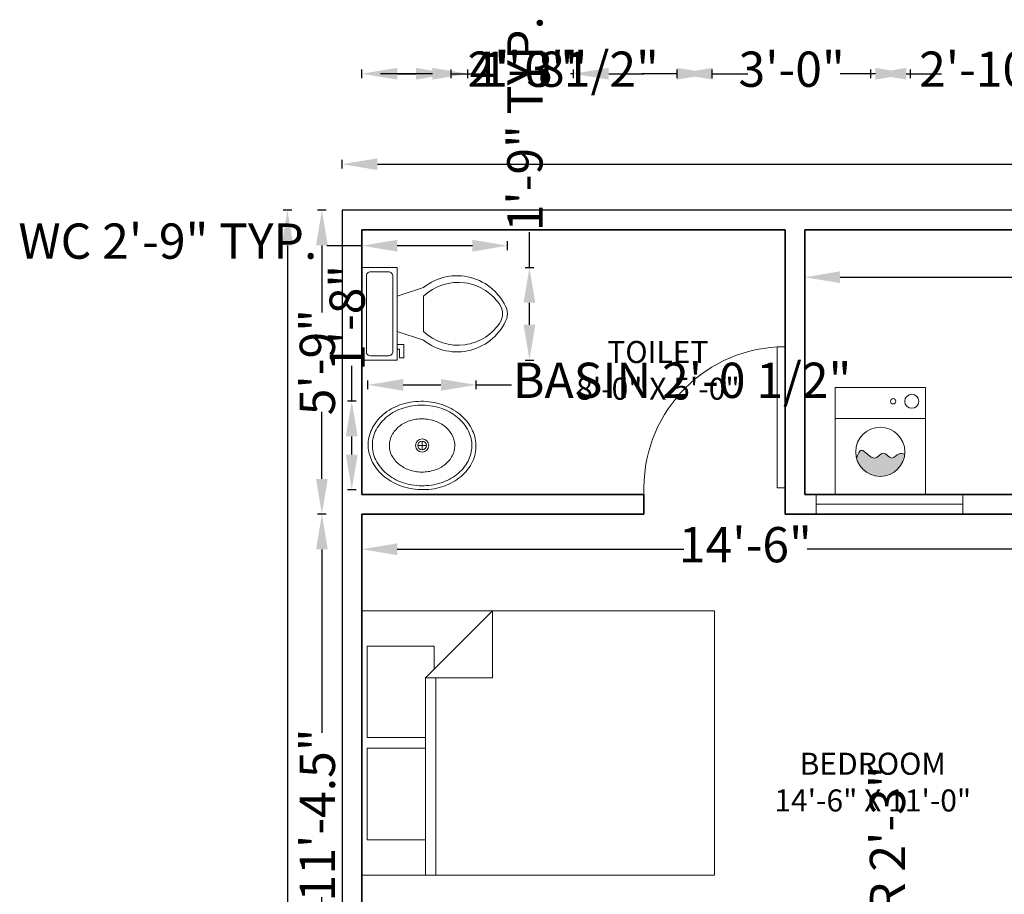
# Model space of a CAD drawing. Units: inches. Extents: x 2174 to 2692, y 577 to 1264.
# Tile 3 of 5: x 2219 to 2442, y 1065 to 1264. Entities that reach past the tile are written whole.
import ezdxf

# ---------------------------------------------------------------- set-up
doc = ezdxf.new("R2010")
doc.units = ezdxf.units.IN
for name, color, linetype, lineweight in [('A-ANNO-DIMS', 2, 'Continuous', 13), ('A-AREA-IDEN', 7, 'Continuous', 18), ('A-DOOR', 3, 'Continuous', 18), ('A-EQPM', 8, 'Continuous', 18), ('A-EQPM-PATT', 8, 'Continuous', 13), ('A-FLOR-FIXT', 9, 'Continuous', 18), ('A-FURN', 8, 'Continuous', 18), ('A-GLAZ', 4, 'Continuous', 18), ('A-WALL', 7, 'Continuous', 35), ('C-PROP', 7, 'Continuous', 25)]:
    doc.layers.add(name, color=color, linetype=linetype, lineweight=lineweight)
doc.styles.get("Standard").update_dxf_attribs({"font": 'arial.ttf'})
doc.dimstyles.new('ISO-25', dxfattribs={"dimtxt": 8, "dimasz": 8, "dimexe": 1, "dimexo": 1, "dimtad": 0, "dimdec": 1, "dimlunit": 3, "dimtxsty": 'Standard', "dimcen": 2.5, "dimclrd": 1, "dimclre": 1, "dimclrt": 1, "dimadec": 0, "dimazin": 0, "dimtfac": 1, "dimtdec": 1, "dimtmove": 0, "dimatfit": 3, "dimfxl": 1, "dimfxlon": 1, "dimarcsym": 0})

# ---------------------------------------------------------------- blocks, each defined once
blk = doc.blocks.new('Bed - Queen')
for p, q in [((0, -80.00003), (0, 0)), ((0, 0), (59.99999, 0)), ((59.99999, 0), (59.99999, -80.00003)), ((7.99999, -1.2), (28.79998, -1.2)), ((7.99999, -14.4), (7.99999, -1.2)), ((28.79998, -1.2), (28.79998, -14.4)), ((31.19999, -1.2), (51.99999, -1.2)), ((31.19999, -14.4), (31.19999, -1.2)), ((51.99999, -1.2), (51.99999, -16.4)), ((0, -14.4), (44.8, -14.4)), ((59.99999, -29.6), (44.8, -14.4)), ((44.8, -14.4), (44.8, -29.6)), ((44.8, -16.8), (0, -16.8)), ((51.99999, -16.4), (46.79936, -16.4)), ((44.8, -29.6), (59.99999, -29.6)), ((59.99999, -80.00003), (0, -80.00003))]:
    blk.add_line(p, q)
blk = doc.blocks.new('Sink - Oval top')
for p, q in [((-1, 0), (1, 0)), ((0, 1), (0, -1))]:
    blk.add_line(p, q)
for points in [[(-12.23, 0.39, 0.117634), (-11.46, -3.36, 0.104469), (-8.88, -6.8, 0.090016), (-5.08, -9.07, 0.08192), (-0.32, -10.02, 0.08192), (4.49, -9.38, 0.090016), (8.42, -7.36, 0.104469), (11.22, -4.09, 0.117634), (12.23, -0.39, 0.117634), (11.46, 3.36, 0.104469), (8.88, 6.8, 0.090016), (5.08, 9.07, 0.08192), (0.32, 10.02, 0.08192), (-4.49, 9.38, 0.090016), (-8.42, 7.36, 0.104469), (-11.22, 4.09, 0.117634)], [(-11.29, 0.16, 0.118622), (-10.52, -3.25, 0.104678), (-8.07, -6.36, 0.089562), (-4.54, -8.37, 0.081185), (-0.13, -9.15, 0.081185), (4.3, -8.49, 0.089562), (7.89, -6.58, 0.104678), (10.42, -3.55, 0.118622), (11.29, -0.16, 0.118622), (10.52, 3.25, 0.104678), (8.07, 6.36, 0.089562), (4.54, 8.37, 0.081185), (0.13, 9.15, 0.081185), (-4.3, 8.49, 0.089562), (-7.89, 6.58, 0.104678), (-10.42, 3.55, 0.118622)], [(-7.42, 0.08, 0.118283), (-6.91, -2.17, 0.104607), (-5.29, -4.21, 0.089718), (-2.97, -5.53, 0.081436), (-0.07, -6.04, 0.081436), (2.84, -5.59, 0.089718), (5.2, -4.33, 0.104607), (6.86, -2.32, 0.118283), (7.42, -0.08, 0.118283), (6.91, 2.17, 0.104607), (5.29, 4.21, 0.089718), (2.97, 5.53, 0.081436), (0.07, 6.04, 0.081436), (-2.84, 5.59, 0.089718), (-5.2, 4.33, 0.104607), (-6.86, 2.32, 0.118283)]]:
    blk.add_lwpolyline(points, format="xyb", close=True)
for radius in [1.5, 1]:
    blk.add_circle((0, 0), radius)
blk = doc.blocks.new('Toilet - top')
for p, q in [((9.5, -6), (9.5, -2)), ((-10, -8.5), (-8, -8.5)), ((-10, -9.5), (-10, -8.5)), ((-8, -8.5), (-8, -8)), ((-7, -8), (-7, -9.5)), ((-4, -8), (-6, -14)), ((4, -8), (6, -14)), ((-7, -9.5), (-10, -9.5)), ((4, -14), (-4, -14))]:
    blk.add_line(p, q)
blk.add_lwpolyline([(10.5, -8), (10.5, 0), (-10.5, 0), (-10.5, -8)], close=True)
for points in [[(-9.5, -2), (-9.5, -6)], [(8.5, -1), (-8.5, -1)], [(-8.5, -7), (8.5, -7)]]:
    blk.add_lwpolyline(points)
for centre, radius, start, end in [((-8.62, -1.88), 0.884, 81.8699, 188.1301), ((8.62, -1.88), 0.884, 351.8699, 98.1301), ((-8.62, -6.12), 0.884, 171.8699, 278.1301), ((8.62, -6.12), 0.884, 261.8699, 8.1301), ((3.52, -21.58), 12.17, 141.4691, 247.9714), ((4.2, -21.82), 11.33, 136.3677, 238.9468), ((-3.52, -21.58), 12.17, 292.0284, 38.5307), ((-4.2, -21.82), 11.33, 301.053, 43.6321), ((0, -27.88), 4, 245.7318, 294.2682), ((0, -29), 4, 254.8605, 285.1395)]:
    blk.add_arc(centre, radius, start, end)
blk = doc.blocks.new('*D9')
at = {"layer": 'A-ANNO-DIMS', "color": 0, "lineweight": -2, "transparency": 16777216}
for p, q in [((2396.95, 1206.12), (2396.95, 1204.12)), ((2404.95, 1205.12), (2470.96, 1205.12)), ((2564.95, 1205.12), (2498.94, 1205.12)), ((2572.95, 1206.12), (2572.95, 1204.12))]:
    blk.add_line(p, q, dxfattribs=at)
at = {"layer": 'A-ANNO-DIMS', "color": 0, "transparency": 16777216}
for points in [[(2404.95, 1206.46), (2404.95, 1203.79), (2396.95, 1205.12)], [(2564.95, 1206.46), (2564.95, 1203.79), (2572.95, 1205.12)]]:
    blk.add_solid(points, dxfattribs=at)
at = {"layer": 'Defpoints', "color": 0, "transparency": 16777216}
for p in [(2396.95, 1215.85), (2572.95, 1215.85), (2396.95, 1205.12)]:
    blk.add_point(p, dxfattribs=at)
at = {"layer": 'A-ANNO-DIMS', "color": 0, "transparency": 16777216, "insert": (2484.95, 1205.12), "char_height": 8, "attachment_point": 5}
blk.add_mtext('14\'-8"', dxfattribs=at)
blk = doc.blocks.new('*D11')
at = {"layer": 'A-ANNO-DIMS', "color": 0, "lineweight": -2, "transparency": 16777216}
for p, q in [((2296.45, 1144.39), (2296.45, 1142.39)), ((2470.45, 1144.39), (2470.45, 1142.39)), ((2304.45, 1143.39), (2369.46, 1143.39)), ((2462.45, 1143.39), (2397.44, 1143.39))]:
    blk.add_line(p, q, dxfattribs=at)
at = {"layer": 'A-ANNO-DIMS', "color": 0, "transparency": 16777216}
for points in [[(2304.45, 1144.72), (2304.45, 1142.05), (2296.45, 1143.39)], [(2462.45, 1144.72), (2462.45, 1142.05), (2470.45, 1143.39)]]:
    blk.add_solid(points, dxfattribs=at)
at = {"layer": 'Defpoints', "color": 0, "transparency": 16777216}
for p in [(2296.45, 1151.35), (2470.45, 1151.35), (2470.45, 1143.39)]:
    blk.add_point(p, dxfattribs=at)
at = {"layer": 'A-ANNO-DIMS', "color": 0, "transparency": 16777216, "insert": (2383.45, 1143.39), "char_height": 8, "attachment_point": 5}
blk.add_mtext('14\'-6"', dxfattribs=at)
blk = doc.blocks.new('*U21')
for p, q in [((0, 0), (0, -6)), ((-32, 0), (-32, -6))]:
    blk.add_line(p, q)
blk.add_lwpolyline([(0, 0), (0, 32), (-1.75, 32), (-1.75, 0)], close=True)
blk.add_arc((0, 0), 32, 90, 180)
blk = doc.blocks.new('*D28')
at = {"layer": 'A-ANNO-DIMS', "color": 0, "lineweight": -2, "transparency": 16777216}
for p, q in [((2291.95, 1229.78), (2291.95, 1231.78)), ((2669.95, 1229.78), (2669.95, 1231.78)), ((2299.95, 1230.78), (2466.59, 1230.78)), ((2661.95, 1230.78), (2495.32, 1230.78))]:
    blk.add_line(p, q, dxfattribs=at)
at = {"layer": 'A-ANNO-DIMS', "color": 0, "transparency": 16777216}
for points in [[(2299.95, 1232.11), (2299.95, 1229.44), (2291.95, 1230.78)], [(2661.95, 1232.11), (2661.95, 1229.44), (2669.95, 1230.78)]]:
    blk.add_solid(points, dxfattribs=at)
at = {"layer": 'Defpoints', "color": 0, "transparency": 16777216}
for p in [(2669.95, 1230.78), (2291.95, 1220.35), (2669.95, 1220.35)]:
    blk.add_point(p, dxfattribs=at)
at = {"layer": 'A-ANNO-DIMS', "color": 0, "transparency": 16777216, "insert": (2480.95, 1230.78), "char_height": 8, "attachment_point": 5}
blk.add_mtext('31\'-6"', dxfattribs=at)
blk = doc.blocks.new('*D29')
at = {"layer": 'A-ANNO-DIMS', "color": 0, "lineweight": -2, "transparency": 16777216}
for p, q in [((2288.37, 1220.35), (2286.37, 1220.35)), ((2287.37, 1212.35), (2287.37, 1197.11)), ((2287.37, 1159.35), (2287.37, 1174.59)), ((2288.37, 1151.35), (2286.37, 1151.35))]:
    blk.add_line(p, q, dxfattribs=at)
at = {"layer": 'A-ANNO-DIMS', "color": 0, "transparency": 16777216}
for points in [[(2286.03, 1212.35), (2288.7, 1212.35), (2287.37, 1220.35)], [(2286.03, 1159.35), (2288.7, 1159.35), (2287.37, 1151.35)]]:
    blk.add_solid(points, dxfattribs=at)
at = {"layer": 'Defpoints', "color": 0, "transparency": 16777216}
for p in [(2291.95, 1220.35), (2287.37, 1151.35), (2291.95, 1151.35)]:
    blk.add_point(p, dxfattribs=at)
at = {"layer": 'A-ANNO-DIMS', "color": 0, "transparency": 16777216, "insert": (2287.37, 1185.85), "char_height": 8, "attachment_point": 5, "rotation": 90}
blk.add_mtext('5\'-9"', dxfattribs=at)
blk = doc.blocks.new('*D30')
at = {"layer": 'A-ANNO-DIMS', "color": 0, "lineweight": -2, "transparency": 16777216}
for p, q in [((2288.37, 1151.35), (2286.37, 1151.35)), ((2287.37, 1143.35), (2287.37, 1101.75)), ((2287.37, 1022.85), (2287.37, 1064.45)), ((2288.37, 1014.85), (2286.37, 1014.85))]:
    blk.add_line(p, q, dxfattribs=at)
at = {"layer": 'A-ANNO-DIMS', "color": 0, "transparency": 16777216}
for points in [[(2286.03, 1143.35), (2288.7, 1143.35), (2287.37, 1151.35)], [(2286.03, 1022.85), (2288.7, 1022.85), (2287.37, 1014.85)]]:
    blk.add_solid(points, dxfattribs=at)
at = {"layer": 'Defpoints', "color": 0, "transparency": 16777216}
for p in [(2291.95, 1151.35), (2287.37, 1014.85), (2296.45, 1014.85)]:
    blk.add_point(p, dxfattribs=at)
at = {"layer": 'A-ANNO-DIMS', "color": 0, "transparency": 16777216, "insert": (2287.37, 1083.1), "char_height": 8, "attachment_point": 5, "rotation": 90}
blk.add_mtext('11\'-4.5"', dxfattribs=at)
blk = doc.blocks.new('*D43')
at = {"layer": 'A-ANNO-DIMS', "color": 0, "lineweight": -2, "transparency": 16777216}
for p, q in [((2280.55, 1220.35), (2278.55, 1220.35)), ((2279.55, 1212.35), (2279.55, 927.77)), ((2279.55, 628.35), (2279.55, 912.94)), ((2280.55, 620.35), (2278.55, 620.35))]:
    blk.add_line(p, q, dxfattribs=at)
at = {"layer": 'A-ANNO-DIMS', "color": 0, "transparency": 16777216}
for points in [[(2278.21, 1212.35), (2280.88, 1212.35), (2279.55, 1220.35)], [(2278.21, 628.35), (2280.88, 628.35), (2279.55, 620.35)]]:
    blk.add_solid(points, dxfattribs=at)
at = {"layer": 'Defpoints', "color": 0, "transparency": 16777216}
for p in [(2291.95, 1220.35), (2279.55, 620.35), (2291.95, 620.35)]:
    blk.add_point(p, dxfattribs=at)
at = {"layer": 'A-ANNO-DIMS', "color": 0, "transparency": 16777216, "insert": (2279.55, 920.35), "char_height": 8, "attachment_point": 5, "rotation": 90}
blk.add_mtext("50'", dxfattribs=at)
blk = doc.blocks.new('*D47')
at = {"layer": 'A-ANNO-DIMS', "color": 1, "lineweight": -2, "transparency": 16777216}
for p, q in [((2296.45, 1211.28), (2296.45, 1213.28)), ((2329.5, 1211.28), (2329.5, 1213.28)), ((2296.45, 1212.28), (2288.45, 1212.28)), ((2321.5, 1212.28), (2304.45, 1212.28))]:
    blk.add_line(p, q, dxfattribs=at)
at = {"layer": 'A-ANNO-DIMS', "color": 1, "transparency": 16777216}
for points in [[(2304.45, 1213.61), (2304.45, 1210.94), (2296.45, 1212.28)], [(2321.5, 1213.61), (2321.5, 1210.94), (2329.5, 1212.28)]]:
    blk.add_solid(points, dxfattribs=at)
at = {"layer": 'Defpoints', "color": 0, "transparency": 16777216}
for p in [(2296.45, 1212.28), (2296.45, 1207.32), (2329.5, 1207.32)]:
    blk.add_point(p, dxfattribs=at)
at = {"layer": 'A-ANNO-DIMS', "color": 1, "transparency": 16777216, "insert": (2252.42, 1212.28), "char_height": 8, "attachment_point": 5}
blk.add_mtext('WC 2\'-9" TYP.', dxfattribs=at)
blk = doc.blocks.new('*D48')
at = {"layer": 'A-ANNO-DIMS', "color": 1, "lineweight": -2, "transparency": 16777216}
for p, q in [((2334.46, 1207.32), (2334.46, 1215.32)), ((2333.46, 1207.32), (2335.46, 1207.32)), ((2334.46, 1194.32), (2334.46, 1199.32)), ((2333.46, 1186.32), (2335.46, 1186.32))]:
    blk.add_line(p, q, dxfattribs=at)
at = {"layer": 'A-ANNO-DIMS', "color": 1, "transparency": 16777216}
for points in [[(2333.12, 1199.32), (2335.79, 1199.32), (2334.46, 1207.32)], [(2333.12, 1194.32), (2335.79, 1194.32), (2334.46, 1186.32)]]:
    blk.add_solid(points, dxfattribs=at)
at = {"layer": 'Defpoints', "color": 0, "transparency": 16777216}
for p in [(2329.5, 1207.32), (2334.46, 1207.32), (2329.5, 1186.32)]:
    blk.add_point(p, dxfattribs=at)
at = {"layer": 'A-ANNO-DIMS', "color": 1, "transparency": 16777216, "insert": (2334.46, 1239.95), "char_height": 8, "attachment_point": 5, "rotation": 90}
blk.add_mtext('1\'-9" TYP.', dxfattribs=at)
blk = doc.blocks.new('*D53')
at = {"layer": 'A-ANNO-DIMS', "color": 1, "lineweight": -2, "transparency": 16777216}
for p, q in [((2416.72, 1015.35), (2416.72, 1023.35)), ((2415.72, 1015.35), (2417.72, 1015.35)), ((2416.72, 996.35), (2416.72, 1007.35)), ((2415.72, 988.35), (2417.72, 988.35))]:
    blk.add_line(p, q, dxfattribs=at)
at = {"layer": 'A-ANNO-DIMS', "color": 1, "transparency": 16777216}
for points in [[(2415.39, 1007.35), (2418.06, 1007.35), (2416.72, 1015.35)], [(2415.39, 996.35), (2418.06, 996.35), (2416.72, 988.35)]]:
    blk.add_solid(points, dxfattribs=at)
at = {"layer": 'Defpoints', "color": 0, "transparency": 16777216}
for p in [(2412.67, 1015.35), (2416.72, 1015.35), (2412.67, 988.35)]:
    blk.add_point(p, dxfattribs=at)
at = {"layer": 'A-ANNO-DIMS', "color": 1, "transparency": 16777216, "insert": (2416.72, 1059.86), "char_height": 8, "attachment_point": 5, "rotation": 90}
blk.add_mtext('ROCKER 2\'-3"', dxfattribs=at)
blk = doc.blocks.new('*D57')
at = {"layer": 'A-ANNO-DIMS', "color": 1, "lineweight": -2, "transparency": 16777216}
for p, q in [((2297.82, 1179.69), (2297.82, 1181.69)), ((2305.82, 1180.69), (2314.37, 1180.69)), ((2322.37, 1179.69), (2322.37, 1181.69)), ((2322.37, 1180.69), (2330.37, 1180.69))]:
    blk.add_line(p, q, dxfattribs=at)
at = {"layer": 'A-ANNO-DIMS', "color": 1, "transparency": 16777216}
for points in [[(2305.82, 1182.02), (2305.82, 1179.36), (2297.82, 1180.69)], [(2314.37, 1182.02), (2314.37, 1179.36), (2322.37, 1180.69)]]:
    blk.add_solid(points, dxfattribs=at)
at = {"layer": 'Defpoints', "color": 0, "transparency": 16777216}
for p in [(2322.37, 1180.69), (2297.82, 1177.01), (2322.37, 1177.01)]:
    blk.add_point(p, dxfattribs=at)
at = {"layer": 'A-ANNO-DIMS', "color": 1, "transparency": 16777216, "insert": (2369.1, 1180.69), "char_height": 8, "attachment_point": 5}
blk.add_mtext('BASIN 2\'-0 1/2"', dxfattribs=at)
blk = doc.blocks.new('*D58')
at = {"layer": 'A-ANNO-DIMS', "color": 1, "lineweight": -2, "transparency": 16777216}
for p, q in [((2294.14, 1177.01), (2294.14, 1185.01)), ((2295.14, 1177.01), (2293.14, 1177.01)), ((2294.14, 1164.87), (2294.14, 1169.01)), ((2295.14, 1156.87), (2293.14, 1156.87))]:
    blk.add_line(p, q, dxfattribs=at)
at = {"layer": 'A-ANNO-DIMS', "color": 1, "transparency": 16777216}
for points in [[(2292.81, 1169.01), (2295.47, 1169.01), (2294.14, 1177.01)], [(2292.81, 1164.87), (2295.47, 1164.87), (2294.14, 1156.87)]]:
    blk.add_solid(points, dxfattribs=at)
at = {"layer": 'Defpoints', "color": 0, "transparency": 16777216}
for p in [(2294.14, 1177.01), (2297.82, 1177.01), (2297.82, 1156.87)]:
    blk.add_point(p, dxfattribs=at)
at = {"layer": 'A-ANNO-DIMS', "color": 1, "transparency": 16777216, "insert": (2294.14, 1195.89), "char_height": 8, "attachment_point": 5, "rotation": 90}
blk.add_mtext('1\'-8"', dxfattribs=at)
blk = doc.blocks.new('*D63')
at = {"layer": 'A-ANNO-DIMS', "color": 1, "lineweight": -2, "transparency": 16777216}
for p, q in [((2360.45, 590.4), (2360.45, 588.4)), ((2392.45, 590.4), (2392.45, 588.4)), ((2352.45, 589.4), (2344.45, 589.4)), ((2360.45, 589.4), (2365.13, 589.4)), ((2392.45, 589.4), (2387.78, 589.4)), ((2400.45, 589.4), (2408.45, 589.4))]:
    blk.add_line(p, q, dxfattribs=at)
at = {"layer": 'A-ANNO-DIMS', "color": 1, "transparency": 16777216}
for points in [[(2352.45, 590.74), (2352.45, 588.07), (2360.45, 589.4)], [(2400.45, 590.74), (2400.45, 588.07), (2392.45, 589.4)]]:
    blk.add_solid(points, dxfattribs=at)
at = {"layer": 'Defpoints', "color": 0, "transparency": 16777216}
for p in [(2360.45, 1155.85), (2392.45, 1155.6), (2392.45, 589.4)]:
    blk.add_point(p, dxfattribs=at)
at = {"layer": 'A-ANNO-DIMS', "color": 1, "transparency": 16777216, "insert": (2376.45, 589.4), "char_height": 8, "attachment_point": 5}
blk.add_mtext('2\'-8"', dxfattribs=at)
blk = doc.blocks.new('*D65')
at = {"layer": 'A-ANNO-DIMS', "color": 1, "lineweight": -2, "transparency": 16777216}
for p, q in [((2412.95, 1251.3), (2404.95, 1251.3)), ((2420.95, 1250.3), (2420.95, 1252.3)), ((2420.95, 1251.3), (2423.52, 1251.3)), ((2454.95, 1251.3), (2452.39, 1251.3)), ((2454.95, 1250.3), (2454.95, 1252.3)), ((2462.95, 1251.3), (2470.95, 1251.3))]:
    blk.add_line(p, q, dxfattribs=at)
at = {"layer": 'A-ANNO-DIMS', "color": 1, "transparency": 16777216}
for points in [[(2412.95, 1252.64), (2412.95, 1249.97), (2420.95, 1251.3)], [(2462.95, 1252.64), (2462.95, 1249.97), (2454.95, 1251.3)]]:
    blk.add_solid(points, dxfattribs=at)
at = {"layer": 'Defpoints', "color": 0, "transparency": 16777216}
for p in [(2454.95, 1251.3), (2420.95, 698.35), (2454.95, 698.35)]:
    blk.add_point(p, dxfattribs=at)
at = {"layer": 'A-ANNO-DIMS', "color": 1, "transparency": 16777216, "insert": (2437.95, 1251.3), "char_height": 8, "attachment_point": 5}
blk.add_mtext('2\'-10"', dxfattribs=at)
blk = doc.blocks.new('*D67')
at = {"layer": 'A-ANNO-DIMS', "color": 1, "lineweight": -2, "transparency": 16777216}
for p, q in [((2312.45, 1251.3), (2304.45, 1251.3)), ((2320.45, 1250.3), (2320.45, 1252.3)), ((2320.45, 1251.3), (2321.13, 1251.3)), ((2344.45, 1251.3), (2343.78, 1251.3)), ((2344.45, 1250.3), (2344.45, 1252.3)), ((2352.45, 1251.3), (2360.45, 1251.3))]:
    blk.add_line(p, q, dxfattribs=at)
at = {"layer": 'A-ANNO-DIMS', "color": 1, "transparency": 16777216}
for points in [[(2312.45, 1252.64), (2312.45, 1249.97), (2320.45, 1251.3)], [(2352.45, 1252.64), (2352.45, 1249.97), (2344.45, 1251.3)]]:
    blk.add_solid(points, dxfattribs=at)
at = {"layer": 'Defpoints', "color": 0, "transparency": 16777216}
for p in [(2344.45, 1251.3), (2320.45, 882.85), (2344.45, 882.85)]:
    blk.add_point(p, dxfattribs=at)
at = {"layer": 'A-ANNO-DIMS', "color": 1, "transparency": 16777216, "insert": (2332.45, 1251.3), "char_height": 8, "attachment_point": 5}
blk.add_mtext('2\'-0"', dxfattribs=at)
blk = doc.blocks.new('*D68')
at = {"layer": 'A-ANNO-DIMS', "color": 1, "lineweight": -2, "transparency": 16777216}
for p, q in [((2367.95, 1251.3), (2359.95, 1251.3)), ((2375.95, 1250.3), (2375.95, 1252.3)), ((2375.95, 1251.3), (2382.7, 1251.3)), ((2411.95, 1251.3), (2405.21, 1251.3)), ((2411.95, 1250.3), (2411.95, 1252.3)), ((2419.95, 1251.3), (2427.95, 1251.3))]:
    blk.add_line(p, q, dxfattribs=at)
at = {"layer": 'A-ANNO-DIMS', "color": 1, "transparency": 16777216}
for points in [[(2367.95, 1252.64), (2367.95, 1249.97), (2375.95, 1251.3)], [(2419.95, 1252.64), (2419.95, 1249.97), (2411.95, 1251.3)]]:
    blk.add_solid(points, dxfattribs=at)
at = {"layer": 'Defpoints', "color": 0, "transparency": 16777216}
for p in [(2411.95, 1251.3), (2375.95, 878.35), (2411.95, 878.35)]:
    blk.add_point(p, dxfattribs=at)
at = {"layer": 'A-ANNO-DIMS', "color": 1, "transparency": 16777216, "insert": (2393.95, 1251.3), "char_height": 8, "attachment_point": 5}
blk.add_mtext('3\'-0"', dxfattribs=at)
blk = doc.blocks.new('*D71')
at = {"layer": 'A-ANNO-DIMS', "color": 1, "lineweight": -2, "transparency": 16777216}
for p, q in [((2308.69, 1251.3), (2300.69, 1251.3)), ((2316.69, 1250.3), (2316.69, 1252.3)), ((2316.69, 1251.3), (2321.61, 1251.3)), ((2368.01, 1251.3), (2363.09, 1251.3)), ((2368.01, 1250.3), (2368.01, 1252.3)), ((2376.01, 1251.3), (2384.01, 1251.3))]:
    blk.add_line(p, q, dxfattribs=at)
at = {"layer": 'A-ANNO-DIMS', "color": 1, "transparency": 16777216}
for points in [[(2308.69, 1252.64), (2308.69, 1249.97), (2316.69, 1251.3)], [(2376.01, 1252.64), (2376.01, 1249.97), (2368.01, 1251.3)]]:
    blk.add_solid(points, dxfattribs=at)
at = {"layer": 'Defpoints', "color": 0, "transparency": 16777216}
for p in [(2368.01, 1251.3), (2316.69, 710.35), (2368.01, 710.35)]:
    blk.add_point(p, dxfattribs=at)
at = {"layer": 'A-ANNO-DIMS', "color": 1, "transparency": 16777216, "insert": (2342.35, 1251.3), "char_height": 8, "attachment_point": 5}
blk.add_mtext('4\'-3 1/2"', dxfattribs=at)
blk = doc.blocks.new('*D72')
at = {"layer": 'A-ANNO-DIMS', "color": 1, "lineweight": -2, "transparency": 16777216}
for p, q in [((2296.45, 1250.3), (2296.45, 1252.3)), ((2304.45, 1251.3), (2308.69, 1251.3)), ((2316.69, 1250.3), (2316.69, 1252.3)), ((2316.69, 1251.3), (2324.69, 1251.3))]:
    blk.add_line(p, q, dxfattribs=at)
at = {"layer": 'A-ANNO-DIMS', "color": 1, "transparency": 16777216}
for points in [[(2304.45, 1252.64), (2304.45, 1249.97), (2296.45, 1251.3)], [(2308.69, 1252.64), (2308.69, 1249.97), (2316.69, 1251.3)]]:
    blk.add_solid(points, dxfattribs=at)
at = {"layer": 'Defpoints', "color": 0, "transparency": 16777216}
for p in [(2316.69, 1251.3), (2296.45, 710.35), (2316.69, 710.35)]:
    blk.add_point(p, dxfattribs=at)
at = {"layer": 'A-ANNO-DIMS', "color": 1, "transparency": 16777216, "insert": (2335.57, 1251.3), "char_height": 8, "attachment_point": 5}
blk.add_mtext('1\'-8"', dxfattribs=at)
blk = doc.blocks.new('*D78')
at = {"layer": 'A-ANNO-DIMS', "color": 1, "lineweight": -2, "transparency": 16777216}
for p, q in [((2399.49, 590.4), (2399.49, 588.4)), ((2432.76, 590.4), (2432.76, 588.4)), ((2407.49, 589.4), (2424.76, 589.4)), ((2432.76, 589.4), (2440.76, 589.4))]:
    blk.add_line(p, q, dxfattribs=at)
at = {"layer": 'A-ANNO-DIMS', "color": 1, "transparency": 16777216}
for points in [[(2407.49, 590.74), (2407.49, 588.07), (2399.49, 589.4)], [(2424.76, 590.74), (2424.76, 588.07), (2432.76, 589.4)]]:
    blk.add_solid(points, dxfattribs=at)
at = {"layer": 'Defpoints', "color": 0, "transparency": 16777216}
for p in [(2399.49, 1151.35), (2432.76, 1151.35), (2432.76, 589.4)]:
    blk.add_point(p, dxfattribs=at)
at = {"layer": 'A-ANNO-DIMS', "color": 1, "transparency": 16777216, "insert": (2461.41, 589.4), "char_height": 8, "attachment_point": 5}
blk.add_mtext('2\'-9 1/2"', dxfattribs=at)

msp = doc.modelspace()

# ---------------------------------------------------------------- hatches: boundary and pattern name
at = {"layer": 'A-EQPM-PATT'}
h = msp.add_hatch(color=256, dxfattribs=at)
h.dxf.hatch_style = 1
edge = h.paths.add_edge_path()
edge.add_spline(control_points=[(2419.61, 1164.96), (2419.19, 1165.08), (2418.08, 1165.4), (2416.62, 1163.17), (2414.72, 1166.22), (2412.52, 1162.58), (2409.79, 1167.25), (2408.99, 1164.89), (2408.69, 1164)], knot_values=[0, 0, 0, 0, 1.255367, 3.233002, 5.426973, 7.643028, 11.192458, 13.339691, 13.339691, 13.339691, 13.339691], degree=3, periodic=0)
edge.add_arc((2414.06, 1165.51), 5.58, 195.7257, 354.3191)

# ---------------------------------------------------------------- linework, layer by layer
at = {"layer": 'A-EQPM'}
for p, q in [((2403.79, 1155.85), (2403.79, 1180.08)), ((2403.79, 1180.08), (2424.33, 1180.08)), ((2424.33, 1180.08), (2424.33, 1155.85)), ((2403.79, 1173.03), (2424.33, 1173.03))]:
    msp.add_line(p, q, dxfattribs=at)
for centre, radius in [((2416.99, 1176.96), 0.603), ((2421.21, 1176.96), 1.59), ((2414.06, 1165.51), 5.58)]:
    msp.add_circle(centre, radius, dxfattribs=at)
msp.add_open_spline([(2408.69, 1164), (2408.99, 1164.89), (2409.79, 1167.25), (2412.52, 1162.58), (2414.72, 1166.22), (2416.62, 1163.17), (2418.08, 1165.4), (2419.19, 1165.08), (2419.61, 1164.96)], degree=3, knots=[0, 0, 0, 0, 2.147233, 5.696662, 7.912718, 10.106688, 12.084324, 13.339691, 13.339691, 13.339691, 13.339691], dxfattribs=at)
at = {"layer": 'A-GLAZ'}
for p, q in [((2399.49, 1155.85), (2399.49, 1151.35)), ((2432.76, 1155.85), (2432.76, 1151.35)), ((2399.49, 1153.6), (2432.76, 1153.6))]:
    msp.add_line(p, q, dxfattribs=at)
at = {"layer": 'A-WALL'}
for p, q in [((2296.45, 1215.85), (2296.45, 1155.85)), ((2392.45, 1215.85), (2296.45, 1215.85)), ((2392.45, 1215.85), (2392.45, 1151.35)), ((2396.95, 1215.85), (2396.95, 1155.85)), ((2572.95, 1215.85), (2396.95, 1215.85)), ((2360.45, 1155.85), (2296.45, 1155.85)), ((2360.45, 1155.85), (2360.45, 1151.35)), ((2470.45, 1155.85), (2396.95, 1155.85)), ((2296.45, 1151.35), (2296.45, 1019.35)), ((2360.45, 1151.35), (2296.45, 1151.35)), ((2470.45, 1151.35), (2392.45, 1151.35))]:
    msp.add_line(p, q, dxfattribs=at)
at = {"layer": 'C-PROP'}
for p, q in [((2669.95, 1220.35), (2291.95, 1220.35)), ((2291.95, 1220.35), (2291.95, 620.35))]:
    msp.add_line(p, q, dxfattribs=at)

# ---------------------------------------------------------------- block references
at = {"layer": 'A-DOOR'}
msp.add_blockref('*U21', (2392.45, 1157.35), dxfattribs=at)
at = {"layer": 'A-FLOR-FIXT', "rotation": 90}
msp.add_blockref('Toilet - top', (2296.45, 1196.82), dxfattribs=at)
at = {"layer": 'A-FLOR-FIXT'}
msp.add_blockref('Sink - Oval top', (2310.1, 1166.94), dxfattribs=at)
at = {"layer": 'A-FURN', "rotation": 90.0000000000235}
msp.add_blockref('Bed - Queen', (2296.45, 1069.43), dxfattribs=at)

# ---------------------------------------------------------------- texts
at = {"layer": 'A-AREA-IDEN', "char_height": 5, "attachment_point": 1}
for s, width, insert in [('\\pxqc;TOILET\\P8\'-0" X 5\'-0"', 38.1431, (2344.53, 1190.65)), ('\\pxqc;BEDROOM\\P14\'-6" X 11\'-0"', 49.045, (2387.83, 1097.21))]:
    msp.add_mtext_dynamic_manual_height_columns(s, width=width, gutter_width=12.5, heights=[0], dxfattribs=dict(at, insert=insert))

# ---------------------------------------------------------------- dimensions: what is measured, and where the dimension line sits
at = {"layer": 'A-ANNO-DIMS'}
for base, p1, p2, override, picture, middle in [((2368.01, 1251.3), (2316.69, 710.35), (2368.01, 710.35), {"dimdec": 1, "dimlfac": 1, "dimrnd": 0, "dimzin": 1, "dimdsep": 46, "dimlunit": 4, "dimfrac": 2}, '*D71', (2342.35, 1251.3)), ((2316.69, 1251.3), (2296.45, 710.35), (2316.69, 710.35), {"dimdec": 1, "dimlfac": 1, "dimrnd": 0, "dimzin": 1, "dimdsep": 46, "dimlunit": 4, "dimfrac": 2}, '*D72', (2335.57, 1251.3)), ((2344.45, 1251.3), (2320.45, 882.85), (2344.45, 882.85), {"dimdec": 1, "dimlfac": 1, "dimrnd": 0, "dimzin": 1, "dimdsep": 46, "dimlunit": 4, "dimfrac": 2}, '*D67', (2332.45, 1251.3)), ((2411.95, 1251.3), (2375.95, 878.35), (2411.95, 878.35), {"dimdec": 1, "dimlfac": 1, "dimrnd": 0, "dimzin": 1, "dimdsep": 46, "dimlunit": 4, "dimfrac": 2}, '*D68', (2393.95, 1251.3)), ((2454.95, 1251.3), (2420.95, 698.35), (2454.95, 698.35), {"dimdec": 1, "dimlfac": 1, "dimrnd": 0, "dimzin": 1, "dimdsep": 46, "dimlunit": 4, "dimfrac": 2}, '*D65', (2437.95, 1251.3)), ((2669.95, 1230.78), (2291.95, 1220.35), (2669.95, 1220.35), {"dimclrd": 0, "dimclre": 0, "dimclrt": 0}, '*D28', (2480.95, 1230.78)), ((2396.95, 1205.12), (2572.95, 1215.85), (2396.95, 1215.85), {"dimclrd": 0, "dimclre": 0, "dimclrt": 0}, '*D9', (2484.95, 1205.12)), ((2392.45, 589.4), (2360.45, 1155.85), (2392.45, 1155.6), {"dimdec": 1, "dimlfac": 1, "dimrnd": 0, "dimzin": 1, "dimdsep": 46, "dimlunit": 4, "dimfrac": 2}, '*D63', (2376.45, 589.4)), ((2432.76, 589.4), (2399.49, 1151.35), (2432.76, 1151.35), {"dimdec": 1, "dimlfac": 1, "dimrnd": 0, "dimzin": 1, "dimdsep": 46, "dimlunit": 4, "dimfrac": 2}, '*D78', (2461.41, 589.4))]:
    dim = msp.add_linear_dim(base=base, p1=p1, p2=p2, dimstyle='ISO-25', override=override, dxfattribs=at)
    dim.commit()
    dim.dimension.update_dxf_attribs({"geometry": picture, "text_midpoint": middle})
for base, p1, p2, angle, text, picture, middle in [((2334.46, 1207.32), (2329.5, 1186.32), (2329.5, 1207.32), 90, '<> TYP.', '*D48', (2334.46, 1239.95)), ((2296.4534, 1212.2768), (2329.4996, 1207.3199), (2296.4534, 1207.3199), 180, 'WC <> TYP.', '*D47', (2252.4205, 1212.2768)), ((2416.72, 1015.35), (2412.67, 988.35), (2412.67, 1015.35), 90, 'ROCKER <>', '*D53', (2416.72, 1059.86))]:
    dim = msp.add_linear_dim(base=base, p1=p1, p2=p2, angle=angle, text=text, dimstyle='ISO-25', override={"dimdec": 1, "dimlfac": 1, "dimrnd": 0, "dimzin": 1, "dimdsep": 46, "dimlunit": 4, "dimfrac": 2}, dxfattribs=at)
    dim.commit()
    dim.dimension.update_dxf_attribs({"geometry": picture, "text_midpoint": middle})
for base, p1, p2, override, picture, middle in [((2279.55, 620.35), (2291.95, 1220.35), (2291.95, 620.35), {"dimclrd": 0, "dimclre": 0, "dimclrt": 0}, '*D43', (2279.55, 920.35)), ((2287.37, 1151.35), (2291.95, 1220.35), (2291.95, 1151.35), {"dimclrd": 0, "dimclre": 0, "dimclrt": 0}, '*D29', (2287.37, 1185.85)), ((2294.14, 1177.01), (2297.82, 1156.87), (2297.82, 1177.01), {"dimdec": 1, "dimlfac": 1, "dimrnd": 0, "dimzin": 1, "dimdsep": 46, "dimlunit": 4, "dimfrac": 2}, '*D58', (2294.14, 1195.89)), ((2287.37, 1014.85), (2291.95, 1151.35), (2296.45, 1014.85), {"dimclrd": 0, "dimclre": 0, "dimclrt": 0, "dimtmove": 1}, '*D30', (2287.37, 1083.1))]:
    dim = msp.add_linear_dim(base=base, p1=p1, p2=p2, angle=90, dimstyle='ISO-25', override=override, dxfattribs=at)
    dim.commit()
    dim.dimension.update_dxf_attribs({"geometry": picture, "text_midpoint": middle})
dim = msp.add_linear_dim(base=(2322.3723, 1180.6888), p1=(2297.8215, 1177.0062), p2=(2322.3723, 1177.0062), text='BASIN <>', dimstyle='ISO-25', override={"dimdec": 1, "dimlfac": 1, "dimrnd": 0, "dimzin": 1, "dimdsep": 46, "dimlunit": 4, "dimfrac": 2}, dxfattribs=at)
dim.commit()
dim.dimension.update_dxf_attribs({"geometry": '*D57', "text_midpoint": (2369.0956, 1180.6888)})
dim = msp.add_linear_dim(base=(2470.45, 1143.39), p1=(2296.45, 1151.35), p2=(2470.45, 1151.35), dimstyle='ISO-25', override={"dimclrd": 0, "dimclre": 0, "dimclrt": 0}, dxfattribs=at)
dim.commit()
dim.dimension.update_dxf_attribs({"geometry": '*D11', "text_midpoint": (2383.45, 1143.39), "dimtype": 160})

doc.saveas('drawing.dxf')
